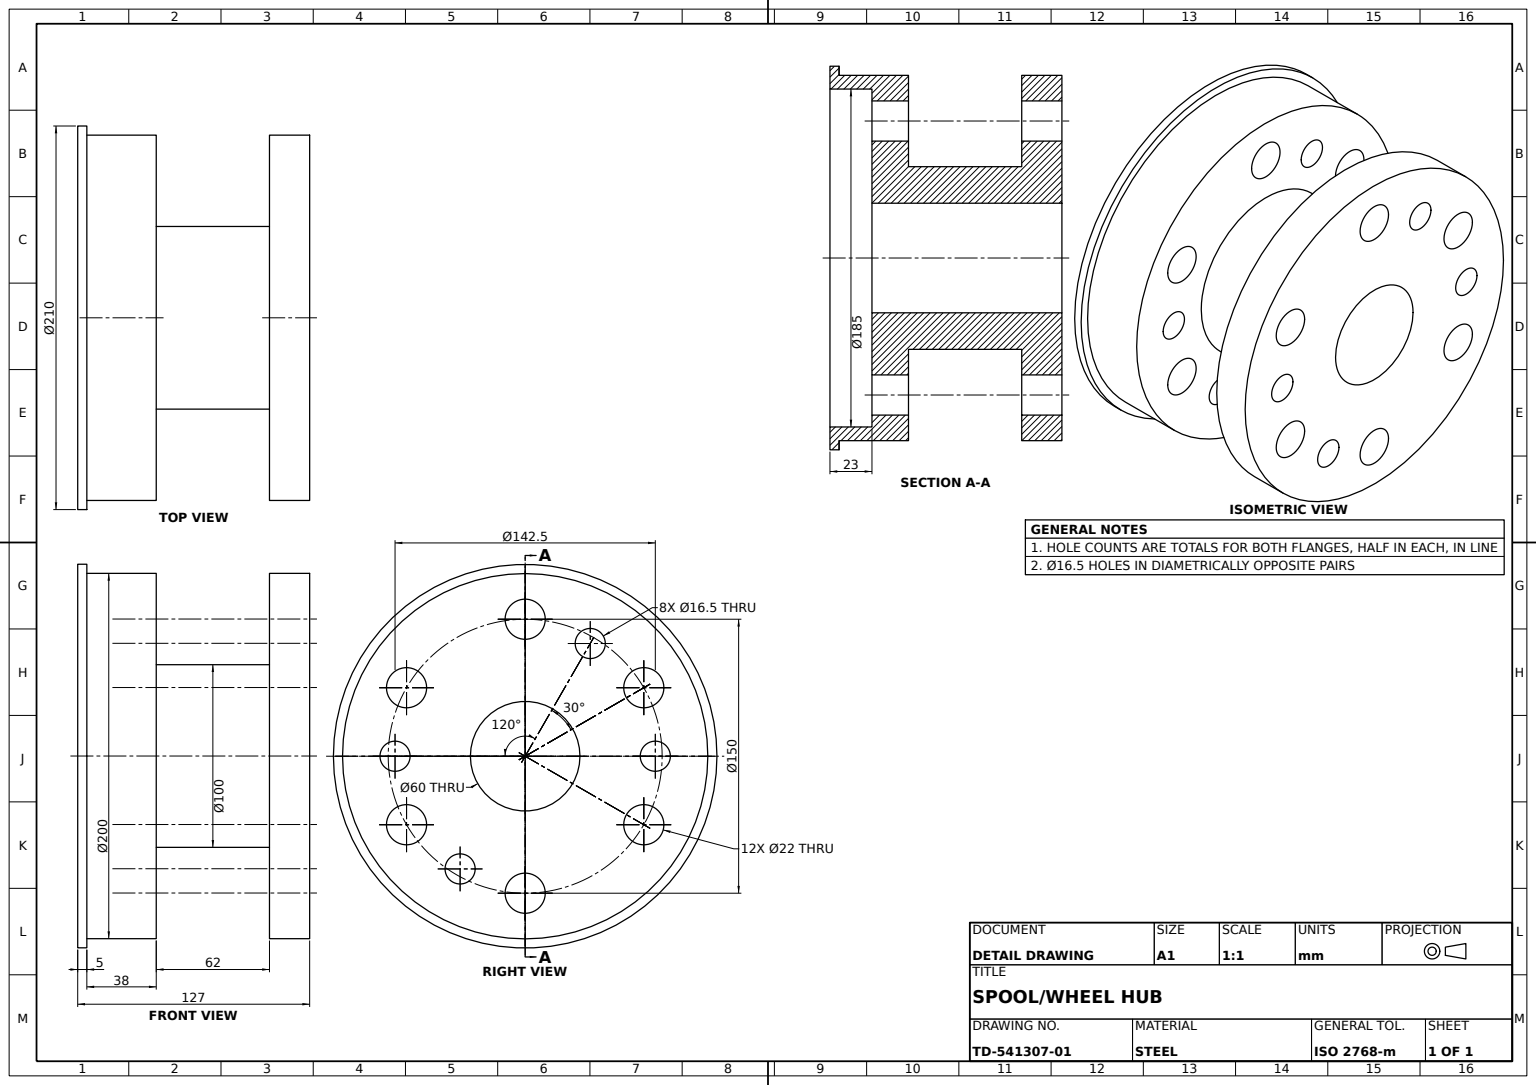
SolidWorks part; units mm, degrees
material "Plain Carbon Steel"
ref_plane "Front Plane" through (0, 0, 0) normal (0, 0, 1) x (1, 0, 0)
ref_plane "Top Plane" through (0, 0, 0) normal (0, 1, 0) x (1, 0, 0)
ref_plane "Right Plane" through (0, 0, 0) normal (1, 0, 0) x (0, 0, -1)
sketch "Rim Lip Sketch Ø210" plane through (0, 0, 0) normal (0, 0, 1) x (1, 0, 0)
  circle A0 centre (0, 0) radius 105
  dimension "D1" = 210
extrude "Rim Lip Ø210" add sketch "Rim Lip Sketch Ø210" against normal blind 5
sketch "Front Flange Sketch Ø200" plane through (0, 0, -5) normal (0, 0, -1) x (-1, 0, 0)
  circle A0 centre (0, 0) radius 100
  dimension "D1" = 200
extrude "Front Flange Ø200" add sketch "Front Flange Sketch Ø200" along normal blind 38
sketch "Hub Barrel Sketch Ø100" plane through (0, 0, -43) normal (0, 0, -1) x (-1, 0, 0)
  circle A0 centre (0, 0) radius 50
  dimension "D1" = 100
extrude "Hub Barrel Ø100" add sketch "Hub Barrel Sketch Ø100" along normal blind 62
sketch "Rear Flange Sketch Ø200" plane through (0, 0, -105) normal (0, 0, -1) x (-1, 0, 0)
  circle A0 centre (0, 0) radius 100
  dimension "D1" = 200
extrude "Rear Flange Ø200" add sketch "Rear Flange Sketch Ø200" along normal blind 22
sketch "Front Recess Sketch Ø185" plane through (0, 0, 0) normal (0, 0, 1) x (1, 0, 0)
  circle A0 centre (0, 0) radius 92.5
  dimension "D1" = 185
extrude "Front Recess Ø185" cut sketch "Front Recess Sketch Ø185" against normal blind 23
sketch "Bore Sketch Ø60" plane through (0, 0, -23) normal (0, 0, 1) x (1, 0, 0)
  circle A0 centre (0, 0) radius 30
  dimension "D1" = 60
extrude "Bore Ø60" cut sketch "Bore Sketch Ø60" against normal through all
sketch "Flange Holes Sketch" plane through (0, 0, -23) normal (0, 0, 1) x (1, 0, 0)
  line L0 (0, 0) -> (-49.9536, 86.5222) construction
  line L1 (0, 0) -> (48.0259, -83.1833) construction
  circle A0 centre (0, 0) radius 75 construction
  circle A1 centre (0, 75) radius 11
  circle A2 centre (64.9519, 37.5) radius 11
  circle A3 centre (64.9519, -37.5) radius 11
  circle A4 centre (0, -75) radius 11
  circle A5 centre (-64.9519, -37.5) radius 11
  circle A6 centre (-64.9519, 37.5) radius 11
  circle A7 centre (0, 0) radius 71.25 construction
  circle A8 centre (-71.25, 0) radius 8.25
  circle A9 centre (71.25, 0) radius 8.25
  circle A11 centre (35.625, -61.7043) radius 8.25
  circle A12 centre (-35.625, 61.7043) radius 8.25
  dimension "D1" = 150
  dimension "D2" = 22
  dimension "D4" = 142.5
  dimension "D5" = 30
  dimension "D7" = 16.5
  dimension "D6" = 30
  dimension "D3" = 6
extrude "Flange Holes" cut sketch "Flange Holes Sketch" against normal through all
